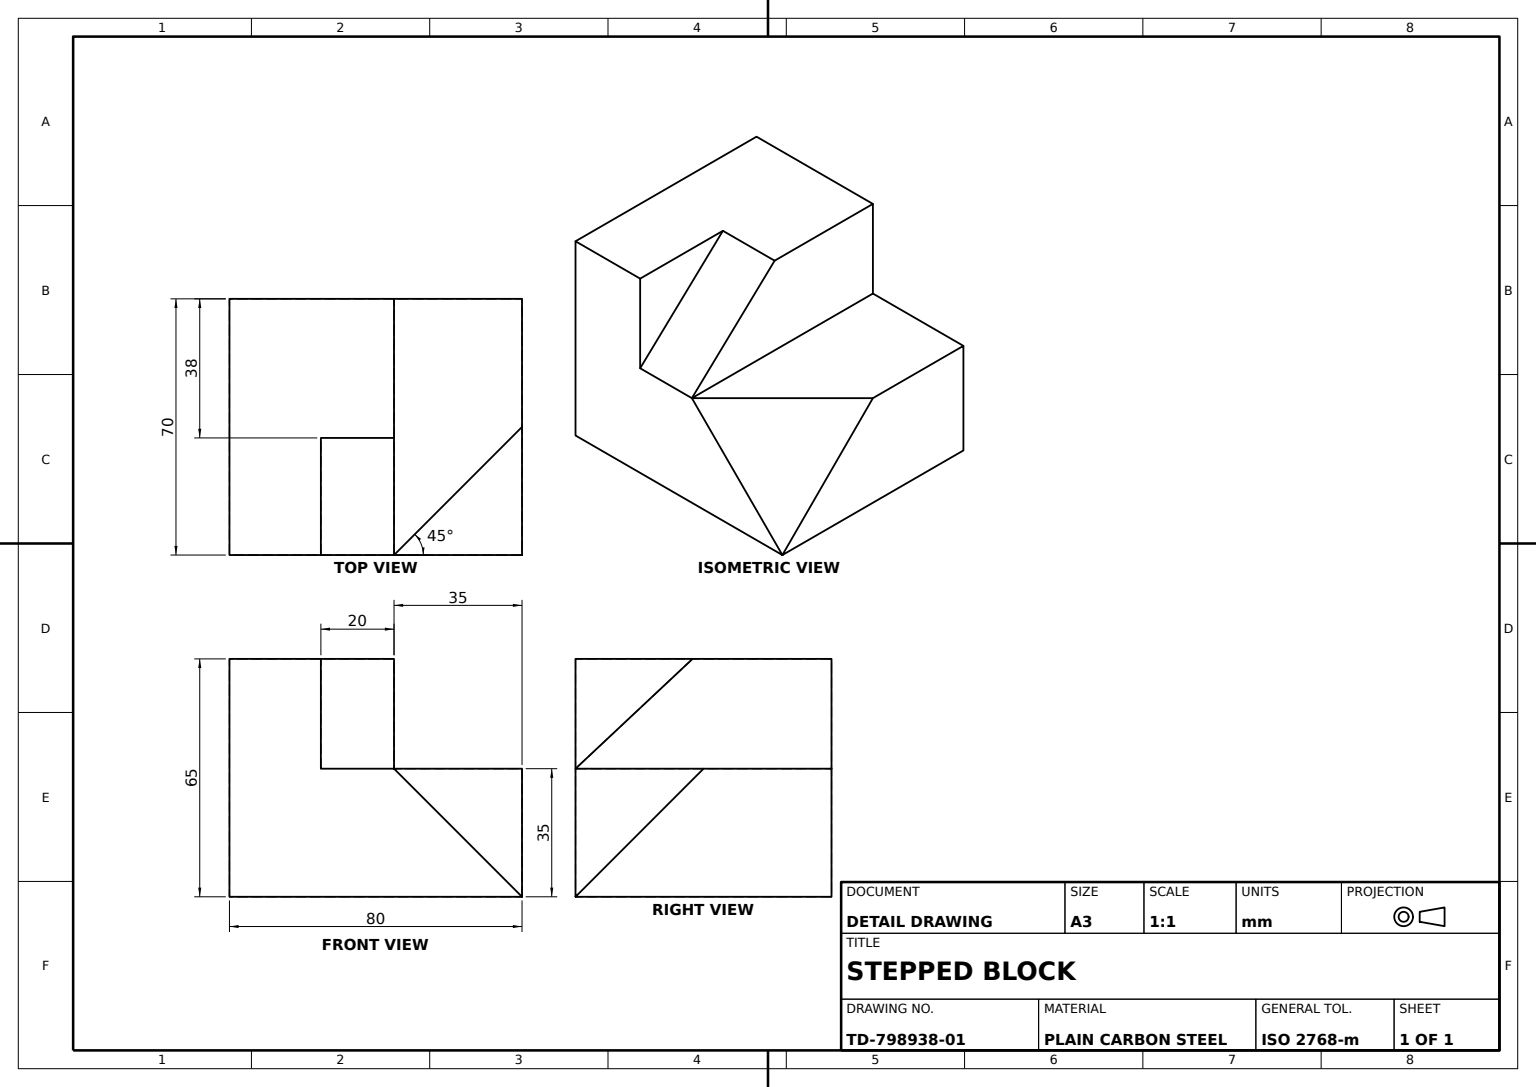
from build123d import *

# Parameters (mm, degrees)
BLOCK_PROFILE_SKETCH_70X65_W = 70
BLOCK_PROFILE_SKETCH_70X65_H = 65
BASE_BLOCK_70X65X80_DEPTH    = 40
UPPER_STEP_SKETCH_W          = 70
UPPER_STEP_SKETCH_H          = 30
UPPER_STEP_CUT_35_DEPTH      = 35
LOWER_STEP_CUT_20_DEPTH      = 20
ANGLED_CORNER_CUT_DEPTH      = 56


with BuildPart() as part:
    # Block Profile Sketch 70x65 → Base Block 70x65x80 (new, symmetric)
    with BuildSketch(Plane.XY):
        with Locations((35, 32.5)):
            Rectangle(BLOCK_PROFILE_SKETCH_70X65_W, BLOCK_PROFILE_SKETCH_70X65_H)
    extrude(amount=BASE_BLOCK_70X65X80_DEPTH, both=True)

    # Upper Step Sketch → Upper Step Cut 35 (cut)
    with BuildSketch(Plane.XY.offset(40)):
        with Locations((35, 50)):
            Rectangle(UPPER_STEP_SKETCH_W, UPPER_STEP_SKETCH_H)
    extrude(amount=-UPPER_STEP_CUT_35_DEPTH, mode=Mode.SUBTRACT)

    # Lower Step Sketch → Lower Step Cut 20 (cut)
    with BuildSketch(Plane.XY.offset(5)):
        Polygon((0, 35), (32, 65), (0, 65), align=None)
    extrude(amount=-LOWER_STEP_CUT_20_DEPTH, mode=Mode.SUBTRACT)

    # Corner Cut Sketch → Angled Corner Cut (cut)
    with BuildSketch(Plane(origin=(-13.333333333, 13.333333333, 13.333333333), x_dir=(-0.8164965809277261, -0.408248290463863, -0.408248290463863), z_dir=(0.5773502691896257, -0.5773502691896258, -0.5773502691896258))):
        Polygon((-16.329931619, 21.213203436), (-16.329931619, -28.284271247), (-59.196002117, -3.535533906), align=None)
    extrude(amount=-ANGLED_CORNER_CUT_DEPTH, mode=Mode.SUBTRACT)


solid = part.part
